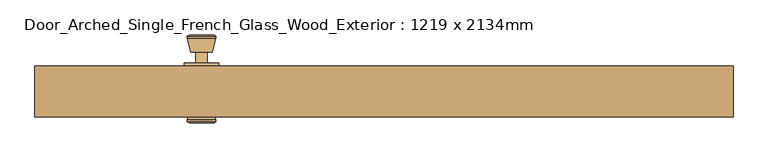
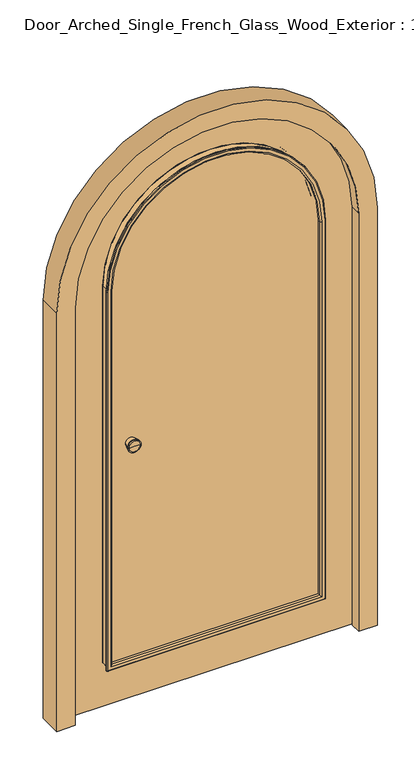
"""IFC4 building model written with IfcOpenShell, lengths in millimetres: door geometry, Door_Arched_Single_French_Glass_Wood_Exterior : 1219 x 2134mm."""

from ifc_helpers import new_model, si_unit, point, frame, frame_2d, origin, place, context, project, spatial, polyline, circle_curve, ellipse_curve, trimmed, segment, composite_curve, outline, extrude, source, transform, mapped, element, save
from ifc_brep_helpers import plane_surface, cylinder_surface, revolved_surface, advanced_brep


def door_arched_single_french_glass_wood_exterior_1219_x_2134mm_67be639c(model_context):
    return source(origin(), model_context, "Body", "SolidModel", [
        advanced_brep(
        [(-318.5, 5.7, 1050.0), (-328.5, 5.7, 1050.0), (-308.5, 5.7, 1050.0), (-298.0241324, 54.7, 1050.0), (-338.9758676, 54.7, 1050.0), (-318.5, 54.7, 1050.0), (-293.5, 52.8721319, 1050.0), (-343.5, 52.8721319, 1050.0), (-293.5, 49.4084537, 1050.0), (-343.5, 49.4084537, 1050.0), (-299.863764, 24.7, 1050.0), (-337.136236, 24.7, 1050.0), (-308.5, 24.7, 1050.0), (-328.5, 24.7, 1050.0)],
        [
            (0, 1),
            (1, 2, circle_curve(frame((-318.5, 5.7, 1050.0), z_axis=(0.0, -1.0, 0.0), x_axis=(-1.0, 0.0, 0.0)), 10.0)),
            (2, 0),
            (2, 1, circle_curve(frame((-318.5, 5.7, 1050.0), z_axis=(0.0, -1.0, 0.0), x_axis=(-1.0, 0.0, 0.0)), 10.0)),
            (3, 4, circle_curve(frame((-318.5, 54.7, 1050.0), z_axis=(0.0, 1.0, 0.0), x_axis=(-1.0, 0.0, 0.0)), 20.4758676)),
            (4, 5),
            (5, 3),
            (4, 3, circle_curve(frame((-318.5, 54.7, 1050.0), z_axis=(0.0, 1.0, 0.0), x_axis=(-1.0, 0.0, 0.0)), 20.4758676)),
            (6, 7, circle_curve(frame((-318.5, 52.8721319, 1050.0), z_axis=(0.0, 1.0, 0.0), x_axis=(-1.0, 0.0, 0.0)), 25.0)),
            (7, 4),
            (3, 6),
            (7, 6, circle_curve(frame((-318.5, 52.8721319, 1050.0), z_axis=(0.0, 1.0, 0.0), x_axis=(-1.0, 0.0, 0.0)), 25.0)),
            (8, 9, circle_curve(frame((-318.5, 49.4084537, 1050.0), z_axis=(0.0, 1.0, 0.0), x_axis=(-1.0, 0.0, 0.0)), 25.0)),
            (9, 7),
            (6, 8),
            (9, 8, circle_curve(frame((-318.5, 49.4084537, 1050.0), z_axis=(0.0, 1.0, 0.0), x_axis=(-1.0, 0.0, 0.0)), 25.0)),
            (10, 11, circle_curve(frame((-318.5, 24.7, 1050.0), z_axis=(0.0, 1.0, 0.0), x_axis=(-1.0, 0.0, 0.0)), 18.636236)),
            (11, 9),
            (8, 10),
            (11, 10, circle_curve(frame((-318.5, 24.7, 1050.0), z_axis=(0.0, 1.0, 0.0), x_axis=(-1.0, 0.0, 0.0)), 18.636236)),
            (12, 13, circle_curve(frame((-318.5, 24.7, 1050.0), z_axis=(0.0, 1.0, 0.0), x_axis=(-1.0, 0.0, 0.0)), 10.0)),
            (13, 11),
            (10, 12),
            (13, 12, circle_curve(frame((-318.5, 24.7, 1050.0), z_axis=(0.0, 1.0, 0.0), x_axis=(-1.0, 0.0, 0.0)), 10.0)),
            (1, 13),
            (12, 2),
        ],
        [
            plane_surface(frame((-318.5, 5.7, 1050.0), z_axis=(0.0, -1.0, 0.0), x_axis=(-1.0, 0.0, 0.0))),
            plane_surface(frame((-318.5, 54.7, 1050.0), z_axis=(0.0, 1.0, 0.0), x_axis=(-1.0, 0.0, 0.0))),
            revolved_surface(polyline([(-338.9758676, 54.7, 1050.0), (-343.5, 52.8721319, 1050.0)]), (-318.5, 5.7, 1050.0), (0.0, -1.0, 0.0)),
            cylinder_surface(frame((-318.5, 5.7, 1050.0), z_axis=(0.0, -1.0, 0.0), x_axis=(-1.0, 0.0, 0.0)), 25.0),
            revolved_surface(polyline([(-343.5, 49.4084537, 1050.0), (-337.136236, 24.7, 1050.0)]), (-318.5, 5.7, 1050.0), (0.0, -1.0, 0.0)),
            plane_surface(frame((-318.5, 24.7, 1050.0), z_axis=(0.0, -1.0, 0.0), x_axis=(-1.0, 0.0, 0.0))),
            cylinder_surface(frame((-318.5, 5.7, 1050.0), z_axis=(0.0, -1.0, 0.0), x_axis=(-1.0, 0.0, 0.0)), 10.0),
        ],
        [
            (0, [[1, 2, 3]]),
            (0, [[-3, 4, -1]]),
            (1, [[5, 6, 7]]),
            (1, [[8, -7, -6]]),
            (2, [[9, 10, -5, 11]]),
            (2, [[12, -11, -8, -10]]),
            (3, [[13, 14, -9, 15]]),
            (3, [[16, -15, -12, -14]]),
            (4, [[17, 18, -13, 19]]),
            (4, [[20, -19, -16, -18]]),
            (5, [[21, 22, -17, 23]]),
            (5, [[24, -23, -20, -22]]),
            (6, [[-2, 25, -21, 26]]),
            (6, [[-4, -26, -24, -25]]),
        ],
    ),
        extrude(outline(composite_curve([segment(trimmed(circle_curve(frame_2d((1050.0, -318.5)), 30.0), [point((1050.0, -348.5))], [point((1050.0, -288.5))], False, "CARTESIAN"), True, "CONTINUOUS"), segment(trimmed(circle_curve(frame_2d((1050.0, -318.5)), 30.0), [point((1050.0, -288.5))], [point((1050.0, -348.5))], False, "CARTESIAN"), True, "CONTINUOUS")], self_intersect=False)), frame((0.0, -0.3, 0.0), z_axis=(0.0, 1.0, 0.0), x_axis=(0.0, 0.0, 1.0)), (0.0, 0.0, 1.0), 6.0),
        advanced_brep(
        [(-318.5, -50.3, 1050.0), (-308.5, -50.3, 1050.0), (-328.5, -50.3, 1050.0), (-298.0241324, -99.3, 1050.0), (-318.5, -99.3, 1050.0), (-338.9758676, -99.3, 1050.0), (-293.5, -97.4721319, 1050.0), (-343.5, -97.4721319, 1050.0), (-293.5, -94.0084537, 1050.0), (-343.5, -94.0084537, 1050.0), (-299.863764, -69.3, 1050.0), (-337.136236, -69.3, 1050.0), (-308.5, -69.3, 1050.0), (-328.5, -69.3, 1050.0)],
        [
            (0, 1),
            (1, 2, circle_curve(frame((-318.5, -50.3, 1050.0), z_axis=(0.0, 1.0, 0.0), x_axis=(-1.0, 0.0, 0.0)), 10.0)),
            (2, 0),
            (2, 1, circle_curve(frame((-318.5, -50.3, 1050.0), z_axis=(0.0, 1.0, 0.0), x_axis=(-1.0, 0.0, 0.0)), 10.0)),
            (3, 4),
            (4, 5),
            (5, 3, circle_curve(frame((-318.5, -99.3, 1050.0), z_axis=(0.0, -1.0, 0.0), x_axis=(-1.0, 0.0, 0.0)), 20.4758676)),
            (3, 5, circle_curve(frame((-318.5, -99.3, 1050.0), z_axis=(0.0, -1.0, 0.0), x_axis=(-1.0, 0.0, 0.0)), 20.4758676)),
            (6, 3),
            (5, 7),
            (7, 6, circle_curve(frame((-318.5, -97.4721319, 1050.0), z_axis=(0.0, -1.0, 0.0), x_axis=(-1.0, 0.0, 0.0)), 25.0)),
            (6, 7, circle_curve(frame((-318.5, -97.4721319, 1050.0), z_axis=(0.0, -1.0, 0.0), x_axis=(-1.0, 0.0, 0.0)), 25.0)),
            (8, 6),
            (7, 9),
            (9, 8, circle_curve(frame((-318.5, -94.0084537, 1050.0), z_axis=(0.0, -1.0, 0.0), x_axis=(-1.0, 0.0, 0.0)), 25.0)),
            (8, 9, circle_curve(frame((-318.5, -94.0084537, 1050.0), z_axis=(0.0, -1.0, 0.0), x_axis=(-1.0, 0.0, 0.0)), 25.0)),
            (10, 8),
            (9, 11),
            (11, 10, circle_curve(frame((-318.5, -69.3, 1050.0), z_axis=(0.0, -1.0, 0.0), x_axis=(-1.0, 0.0, 0.0)), 18.636236)),
            (10, 11, circle_curve(frame((-318.5, -69.3, 1050.0), z_axis=(0.0, -1.0, 0.0), x_axis=(-1.0, 0.0, 0.0)), 18.636236)),
            (12, 10),
            (11, 13),
            (13, 12, circle_curve(frame((-318.5, -69.3, 1050.0), z_axis=(0.0, -1.0, 0.0), x_axis=(-1.0, 0.0, 0.0)), 10.0)),
            (12, 13, circle_curve(frame((-318.5, -69.3, 1050.0), z_axis=(0.0, -1.0, 0.0), x_axis=(-1.0, 0.0, 0.0)), 10.0)),
            (1, 12),
            (13, 2),
        ],
        [
            plane_surface(frame((-318.5, -50.3, 1050.0), z_axis=(0.0, 1.0, 0.0), x_axis=(-1.0, 0.0, 0.0))),
            plane_surface(frame((-318.5, -99.3, 1050.0), z_axis=(0.0, -1.0, 0.0), x_axis=(-1.0, 0.0, 0.0))),
            revolved_surface(polyline([(-338.9758676, -99.3, 1050.0), (-343.5, -97.4721319, 1050.0)]), (-318.5, -50.3, 1050.0), (0.0, 1.0, 0.0)),
            cylinder_surface(frame((-318.5, -50.3, 1050.0), z_axis=(0.0, 1.0, 0.0), x_axis=(-1.0, 0.0, 0.0)), 25.0),
            revolved_surface(polyline([(-343.5, -94.0084537, 1050.0), (-337.136236, -69.3, 1050.0)]), (-318.5, -50.3, 1050.0), (0.0, 1.0, 0.0)),
            plane_surface(frame((-318.5, -69.3, 1050.0), z_axis=(0.0, 1.0, 0.0), x_axis=(-1.0, 0.0, 0.0))),
            cylinder_surface(frame((-318.5, -50.3, 1050.0), z_axis=(0.0, 1.0, 0.0), x_axis=(-1.0, 0.0, 0.0)), 10.0),
        ],
        [
            (0, [[1, 2, 3]]),
            (0, [[-3, 4, -1]]),
            (1, [[5, 6, 7]]),
            (1, [[-6, -5, 8]]),
            (2, [[9, -7, 10, 11]]),
            (2, [[-10, -8, -9, 12]]),
            (3, [[13, -11, 14, 15]]),
            (3, [[-14, -12, -13, 16]]),
            (4, [[17, -15, 18, 19]]),
            (4, [[-18, -16, -17, 20]]),
            (5, [[21, -19, 22, 23]]),
            (5, [[-22, -20, -21, 24]]),
            (6, [[25, -23, 26, -2]]),
            (6, [[-26, -24, -25, -4]]),
        ],
    ),
        extrude(outline(composite_curve([segment(trimmed(circle_curve(frame_2d((1050.0, -318.5)), 30.0), [point((1050.0, -348.5))], [point((1050.0, -288.5))], False, "CARTESIAN"), True, "CONTINUOUS"), segment(trimmed(circle_curve(frame_2d((1050.0, -318.5)), 30.0), [point((1050.0, -288.5))], [point((1050.0, -348.5))], False, "CARTESIAN"), True, "CONTINUOUS")], self_intersect=False)), frame((0.0, -50.3, 0.0), z_axis=(0.0, 1.0, 0.0), x_axis=(0.0, 0.0, 1.0)), (0.0, 0.0, 1.0), 6.0),
        advanced_brep(
        [(539.1, -89.3, 0.0), (539.1, -47.3, 0.0), (561.1, -47.3, 0.0), (561.1, -0.3, 0.0), (609.6, -0.3, 0.0), (609.6, -89.3, 0.0), (609.6, -89.3, 1678.6), (-609.6, -89.3, 1678.6), (-609.6, -89.3, 0.0), (-539.1, -89.3, 0.0), (-539.1, -89.3, 1678.6), (539.1, -89.3, 1678.6), (609.6, -0.3, 1678.6), (561.1, -0.3, 1678.6), (-561.1, -0.3, 1678.6), (-561.1, -0.3, 0.0), (-609.6, -0.3, 0.0), (-609.6, -0.3, 1678.6), (561.1, -47.3, 1678.6), (539.1, -47.3, 1678.6), (-539.1, -47.3, 1678.6), (-539.1, -47.3, 0.0), (-561.1, -47.3, 0.0), (-561.1, -47.3, 1678.6)],
        [
            (0, 1),
            (1, 2),
            (2, 3),
            (3, 4),
            (4, 5),
            (5, 0),
            (5, 6),
            (6, 7, circle_curve(frame((0.0, -89.3, 1678.6), z_axis=(0.0, -1.0, 0.0), x_axis=(1.0, 0.0, 0.0)), 609.6)),
            (7, 8),
            (8, 9),
            (9, 10),
            (10, 11, circle_curve(frame((0.0, -89.3, 1678.6), z_axis=(0.0, 1.0, 0.0), x_axis=(1.0, 0.0, 0.0)), 539.1)),
            (11, 0),
            (4, 12),
            (12, 6),
            (3, 13),
            (13, 14, circle_curve(frame((0.0, -0.3, 1678.6), z_axis=(0.0, -1.0, 0.0), x_axis=(1.0, 0.0, 0.0)), 561.1)),
            (14, 15),
            (15, 16),
            (16, 17),
            (17, 12, circle_curve(frame((0.0, -0.3, 1678.6), z_axis=(0.0, 1.0, 0.0), x_axis=(1.0, 0.0, 0.0)), 609.6)),
            (2, 18),
            (18, 13),
            (1, 19),
            (19, 20, circle_curve(frame((0.0, -47.3, 1678.6), z_axis=(0.0, -1.0, 0.0), x_axis=(1.0, 0.0, 0.0)), 539.1)),
            (20, 21),
            (21, 22),
            (22, 23),
            (23, 18, circle_curve(frame((0.0, -47.3, 1678.6), z_axis=(0.0, 1.0, 0.0), x_axis=(1.0, 0.0, 0.0)), 561.1)),
            (11, 19),
            (9, 21),
            (20, 10),
            (8, 16),
            (15, 22),
            (7, 17),
            (14, 23),
        ],
        [
            plane_surface(frame((603.1, 9.1123976, 0.0), z_axis=(0.0, 0.0, -1.0), x_axis=(1.0, 0.0, 0.0))),
            plane_surface(frame((539.1, -89.3, 0.0), z_axis=(0.0, -1.0, 0.0), x_axis=(0.0, 0.0, 1.0))),
            plane_surface(frame((609.6, -89.3, 0.0), z_axis=(1.0, 0.0, 0.0), x_axis=(0.0, 0.0, 1.0))),
            plane_surface(frame((609.6, -0.3, 0.0), z_axis=(0.0, 1.0, 0.0), x_axis=(0.0, 0.0, 1.0))),
            plane_surface(frame((561.1, -0.3, 0.0), z_axis=(-1.0, 0.0, 0.0), x_axis=(0.0, 0.0, 1.0))),
            plane_surface(frame((561.1, -47.3, 0.0), z_axis=(0.0, 1.0, 0.0), x_axis=(0.0, 0.0, 1.0))),
            plane_surface(frame((539.1, -47.3, 0.0), z_axis=(-1.0, 0.0, 0.0), x_axis=(0.0, 0.0, 1.0))),
            plane_surface(frame((-539.1, -47.3, 1678.6), z_axis=(1.0, 0.0, 0.0), x_axis=(0.0, 0.0, -1.0))),
            plane_surface(frame((-603.1, 9.1123976, 0.0), z_axis=(0.0, 0.0, -1.0), x_axis=(-1.0, 0.0, 0.0))),
            plane_surface(frame((-609.6, -89.3, 1678.6), z_axis=(-1.0, 0.0, 0.0), x_axis=(0.0, 0.0, -1.0))),
            plane_surface(frame((-561.1, -0.3, 1678.6), z_axis=(1.0, 0.0, 0.0), x_axis=(0.0, 0.0, -1.0))),
            cylinder_surface(frame((0.0, -89.3, 1678.6), z_axis=(0.0, 1.0, 0.0), x_axis=(1.0, 0.0, 0.0)), 609.6),
            revolved_surface(polyline([(561.1, -0.29999999999999716, 1678.6), (561.1, -47.3, 1678.6)]), (0.0, -89.3, 1678.6), (0.0, 1.0, 0.0)),
            revolved_surface(polyline([(539.1, -47.3, 1678.6), (539.1, -89.3, 1678.6)]), (0.0, -89.3, 1678.6), (0.0, 1.0, 0.0)),
        ],
        [
            (0, [[1, 2, 3, 4, 5, 6]]),
            (1, [[7, 8, 9, 10, 11, 12, 13, -6]]),
            (2, [[14, 15, -7, -5]]),
            (3, [[16, 17, 18, 19, 20, 21, -14, -4]]),
            (4, [[22, 23, -16, -3]]),
            (5, [[24, 25, 26, 27, 28, 29, -22, -2]]),
            (6, [[-13, 30, -24, -1]]),
            (7, [[-11, 31, -26, 32]]),
            (8, [[-10, 33, -19, 34, -27, -31]]),
            (9, [[-20, -33, -9, 35]]),
            (10, [[-28, -34, -18, 36]]),
            (11, [[-35, -8, -15, -21]]),
            (12, [[-36, -17, -23, -29]]),
            (13, [[-32, -25, -30, -12]]),
        ],
    ),
        extrude(outline(composite_curve([segment(trimmed(circle_curve(frame_2d((1692.1, 0.0)), 253.5), [point((1896.740356, 149.6147543))], [point((1905.7961472, 136.3679092))], False, "CARTESIAN"), True, "CONTINUOUS"), segment(polyline([(1905.7961472, 136.3679092), (1768.2345335, 56.9466745)]), True, "CONTINUOUS"), segment(trimmed(circle_curve(frame_2d((1653.6, 0.0)), 128.0), [point((1768.2345335, 56.9466745))], [point((1768.2345335, -56.9466745))], False, "CARTESIAN"), True, "CONTINUOUS"), segment(polyline([(1768.2345335, -56.9466745), (1905.7961472, -136.3679092)]), True, "CONTINUOUS"), segment(trimmed(circle_curve(frame_2d((1692.1, 0.0)), 253.5), [point((1905.7961472, -136.3679092))], [point((1896.740356, -149.6147543))], False, "CARTESIAN"), True, "CONTINUOUS"), segment(polyline([(1896.740356, -149.6147543), (1760.2345335, -70.8030809)]), True, "CONTINUOUS"), segment(trimmed(circle_curve(frame_2d((1653.6, 0.0)), 128.0), [point((1760.2345335, -70.8030809))], [point((1661.6, -127.7497554))], False, "CARTESIAN"), True, "CONTINUOUS"), segment(polyline([(1661.6, -127.7497554), (1661.6, -408.1), (1645.6, -408.1), (1645.6, -128.0), (1273.5, -128.0), (1273.5, -408.1), (1257.5, -408.1), (1257.5, -128.0), (909.0, -128.0), (909.0, -408.1), (893.0, -408.1), (893.0, -128.0), (544.5, -128.0), (544.5, -408.1), (528.5, -408.1), (528.5, -128.0), (179.0, -128.0), (179.0, -112.0), (528.5, -112.0), (528.5, 112.0), (179.0, 112.0), (179.0, 128.0), (528.5, 128.0), (528.5, 408.1), (544.5, 408.1), (544.5, 128.0), (893.0, 128.0), (893.0, 408.1), (909.0, 408.1), (909.0, 128.0), (1257.5, 128.0), (1257.5, 408.1), (1273.5, 408.1), (1273.5, 128.0), (1645.6, 128.0), (1645.6, 408.1), (1661.6, 408.1), (1661.6, 127.7497554)]), True, "CONTINUOUS"), segment(trimmed(circle_curve(frame_2d((1653.6, 0.0)), 128.0), [point((1661.6, 127.7497554))], [point((1760.2345335, 70.8030809))], False, "CARTESIAN"), True, "CONTINUOUS"), segment(polyline([(1760.2345335, 70.8030809), (1896.740356, 149.6147543)]), True, "CONTINUOUS")], self_intersect=False), holes=[polyline([(893.0, -112.0), (893.0, 112.0), (544.5, 112.0), (544.5, -112.0), (893.0, -112.0)]), polyline([(1257.5, 112.0), (909.0, 112.0), (909.0, -112.0), (1257.5, -112.0), (1257.5, 112.0)]), composite_curve([segment(trimmed(circle_curve(frame_2d((1653.6, 0.0)), 112.0), [point((1661.6, -111.7139204))], [point((1661.6, 111.7139204))], True, "CARTESIAN"), True, "CONTINUOUS"), segment(polyline([(1661.6, 111.7139204), (1661.6, -111.7139204)]), True, "CONTINUOUS")], self_intersect=False), polyline([(1645.6, -112.0), (1645.6, 112.0), (1273.5, 112.0), (1273.5, -112.0), (1645.6, -112.0)])]), frame((0.0, -29.6874553, 0.0), z_axis=(0.0, 1.0, 0.0), x_axis=(0.0, 0.0, 1.0)), (0.0, 0.0, 1.0), 14.5359085),
        extrude(outline(composite_curve([segment(polyline([(4.0, 558.1), (1727.8950302, 558.1)]), True, "CONTINUOUS"), segment(trimmed(circle_curve(frame_2d((1678.6, 0.0)), 560.2727996), [point((1727.8950302, 558.1))], [point((1715.9714663, -559.0250294))], False, "CARTESIAN"), True, "CONTINUOUS"), segment(polyline([(1715.9714663, -559.0250294), (4.0, -559.0250294), (4.0, 558.1)]), True, "CONTINUOUS")], self_intersect=False), holes=[composite_curve([segment(polyline([(179.0, -408.1), (1692.1, -408.1)]), True, "CONTINUOUS"), segment(trimmed(circle_curve(frame_2d((1692.1, 0.0)), 408.1), [point((1692.1, -408.1))], [point((1692.1, 408.1))], True, "CARTESIAN"), True, "CONTINUOUS"), segment(polyline([(1692.1, 408.1), (179.0, 408.1), (179.0, -408.1)]), True, "CONTINUOUS")], self_intersect=False)]), frame((0.0, -44.3, 0.0), z_axis=(0.0, 1.0, 0.0), x_axis=(0.0, 0.0, 1.0)), (0.0, 0.0, 1.0), 44.0),
        extrude(outline(composite_curve([segment(polyline([(179.0, -408.1), (179.0, 408.1), (1692.1, 408.1)]), True, "CONTINUOUS"), segment(trimmed(circle_curve(frame_2d((1692.1, 0.0)), 408.1), [point((1692.1, 408.1))], [point((1692.1, -408.1))], False, "CARTESIAN"), True, "CONTINUOUS"), segment(polyline([(1692.1, -408.1), (179.0, -408.1)]), True, "CONTINUOUS")], self_intersect=False)), frame((0.0, -70.0, 0.0), z_axis=(0.0, 1.0, 0.0), x_axis=(0.0, 0.0, 1.0)), (0.0, 0.0, 1.0), 24.0),
        advanced_brep(
        [(-416.1, -84.0, 171.0), (-416.1, -84.0, 1692.1), (-416.1, -80.0, 1692.1), (-416.1, -80.0, 171.0), (-414.1, -86.0, 173.0), (-414.1, -86.0, 1692.1), (-396.1, -81.0, 191.0), (-396.1, -81.0, 1692.1), (-401.1, -86.0, 1692.1), (-401.1, -86.0, 186.0), (-396.1, -70.0, 191.0), (-396.1, -70.0, 1692.1), (-408.1, -80.0, 179.0), (-408.1, -80.0, 1692.1), (-408.1, -70.0, 1692.1), (-408.1, -70.0, 179.0), (416.1, -84.0, 1692.1), (416.1, -80.0, 1692.1), (414.1, -86.0, 1692.1), (414.1, -86.0, 173.0), (401.1, -86.0, 1692.1), (401.1, -86.0, 186.0), (396.1, -81.0, 1692.1), (396.1, -70.0, 1692.1), (408.1, -70.0, 1692.1), (408.1, -70.0, 179.0), (396.1, -70.0, 191.0), (408.1, -80.0, 1692.1), (416.1, -80.0, 171.0), (408.1, -80.0, 179.0), (416.1, -84.0, 171.0), (396.1, -81.0, 191.0)],
        [
            (0, 1),
            (1, 2),
            (2, 3),
            (3, 0),
            (4, 5),
            (5, 1, circle_curve(frame((-414.1, -84.0, 1692.1), z_axis=(0.0, 0.0, -1.0), x_axis=(-1.0, 0.0, 0.0)), 2.0)),
            (0, 4, ellipse_curve(frame((-414.1, -84.0, 173.0), z_axis=(-0.7071067811865475, 0.0, 0.7071067811865475), x_axis=(-0.7071067811865474, 0.0, -0.7071067811865476)), 2.8284271, 2.0)),
            (6, 7),
            (7, 8, circle_curve(frame((-401.1, -81.0, 1692.1), z_axis=(0.0, 0.0, -1.0), x_axis=(-1.0, 0.0, 0.0)), 5.0)),
            (8, 9),
            (9, 6, ellipse_curve(frame((-401.1, -81.0, 186.0), z_axis=(-0.7071067811865475, 0.0, 0.7071067811865475), x_axis=(-0.7071067811865474, 0.0, -0.7071067811865476)), 7.0710678, 5.0)),
            (10, 11),
            (11, 7),
            (6, 10),
            (12, 13),
            (13, 14),
            (14, 15),
            (15, 12),
            (16, 17),
            (17, 2, circle_curve(frame((0.0, -80.0, 1692.1), z_axis=(0.0, -1.0, 0.0), x_axis=(-1.0, 0.0, 0.0)), 416.1)),
            (1, 16, circle_curve(frame((0.0, -84.0, 1692.1), z_axis=(0.0, 1.0, 0.0), x_axis=(-1.0, 0.0, 0.0)), 416.1)),
            (18, 16, circle_curve(frame((414.1, -84.0, 1692.1), z_axis=(0.0, 0.0, 1.0), x_axis=(1.0, 0.0, 0.0)), 2.0)),
            (5, 18, circle_curve(frame((0.0, -86.0, 1692.1), z_axis=(0.0, 1.0, 0.0), x_axis=(-1.0, 0.0, 0.0)), 414.1)),
            (4, 19),
            (19, 18),
            (20, 21),
            (21, 9),
            (8, 20, circle_curve(frame((0.0, -86.0, 1692.1), z_axis=(0.0, 1.0, 0.0), x_axis=(-1.0, 0.0, 0.0)), 401.1)),
            (22, 20, circle_curve(frame((401.1, -81.0, 1692.1), z_axis=(0.0, 0.0, 1.0), x_axis=(1.0, 0.0, 0.0)), 5.0)),
            (7, 22, circle_curve(frame((0.0, -81.0, 1692.1), z_axis=(0.0, 1.0, 0.0), x_axis=(-1.0, 0.0, 0.0)), 396.1)),
            (23, 22),
            (11, 23, circle_curve(frame((0.0, -70.0, 1692.1), z_axis=(0.0, 1.0, 0.0), x_axis=(-1.0, 0.0, 0.0)), 396.1)),
            (24, 25),
            (25, 15),
            (14, 24, circle_curve(frame((0.0, -70.0, 1692.1), z_axis=(0.0, 1.0, 0.0), x_axis=(-1.0, 0.0, 0.0)), 408.1)),
            (10, 26),
            (26, 23),
            (27, 24),
            (13, 27, circle_curve(frame((0.0, -80.0, 1692.1), z_axis=(0.0, 1.0, 0.0), x_axis=(-1.0, 0.0, 0.0)), 408.1)),
            (17, 28),
            (28, 3),
            (12, 29),
            (29, 27),
            (16, 30),
            (30, 28),
            (19, 30, ellipse_curve(frame((414.1, -84.0, 173.0), z_axis=(0.7071067811865475, 0.0, 0.7071067811865475), x_axis=(-0.7071067811865474, 0.0, 0.7071067811865476)), 2.8284271, 2.0)),
            (22, 31),
            (31, 21, ellipse_curve(frame((401.1, -81.0, 186.0), z_axis=(0.7071067811865475, 0.0, 0.7071067811865475), x_axis=(-0.7071067811865474, 0.0, 0.7071067811865476)), 7.0710678, 5.0)),
            (26, 31),
            (29, 25),
            (30, 0),
            (31, 6),
        ],
        [
            plane_surface(frame((-416.1, -80.0, 171.0), z_axis=(-1.0, 0.0, 0.0), x_axis=(0.0, 0.0, 1.0))),
            cylinder_surface(frame((-414.1, -84.0, 179.0), z_axis=(0.0, 0.0, -1.0), x_axis=(-1.0, 0.0, 0.0)), 2.0),
            cylinder_surface(frame((-401.1, -81.0, 179.0), z_axis=(0.0, 0.0, -1.0), x_axis=(-1.0, 0.0, 0.0)), 5.0),
            plane_surface(frame((-396.1, -81.0, 191.0), z_axis=(1.0, 0.0, 0.0), x_axis=(0.0, 0.0, 1.0))),
            plane_surface(frame((-408.1, -70.0, 179.0), z_axis=(-1.0, 0.0, 0.0), x_axis=(0.0, 0.0, 1.0))),
            cylinder_surface(frame((0.0, -80.0, 1692.1), z_axis=(0.0, -1.0, 0.0), x_axis=(-1.0, 0.0, 0.0)), 416.1),
            revolved_surface(trimmed(ellipse_curve(frame((-414.1, -84.0, 1692.1), z_axis=(0.0, 0.0, 1.0), x_axis=(-1.0, 0.0, 0.0)), 2.0, 2.0), [point((-416.1, -84.0, 1692.1))], [point((-414.1, -86.0, 1692.1))], True, "CARTESIAN"), (0.0, -80.0, 1692.1), (0.0, -1.0, 0.0)),
            plane_surface(frame((0.0, -86.0, 1692.1), z_axis=(0.0, -1.0, 0.0), x_axis=(-1.0, 0.0, 0.0))),
            revolved_surface(trimmed(ellipse_curve(frame((-401.1, -81.0, 1692.1), z_axis=(0.0, 0.0, 1.0), x_axis=(-1.0, 0.0, 0.0)), 5.0, 5.0), [point((-401.1, -86.0, 1692.1))], [point((-396.1, -81.0, 1692.1))], True, "CARTESIAN"), (0.0, -80.0, 1692.1), (0.0, -1.0, 0.0)),
            revolved_surface(polyline([(-396.1, -81.0, 1692.1), (-396.1, -70.0, 1692.1)]), (0.0, -80.0, 1692.1), (0.0, -1.0, 0.0)),
            plane_surface(frame((0.0, -70.0, 1692.1), z_axis=(0.0, 1.0, 0.0), x_axis=(-1.0, 0.0, 0.0))),
            cylinder_surface(frame((0.0, -80.0, 1692.1), z_axis=(0.0, -1.0, 0.0), x_axis=(-1.0, 0.0, 0.0)), 408.1),
            plane_surface(frame((0.0, -80.0, 1692.1), z_axis=(0.0, 1.0, 0.0), x_axis=(-1.0, 0.0, 0.0))),
            plane_surface(frame((416.1, -80.0, 1692.1), z_axis=(1.0, 0.0, 0.0), x_axis=(0.0, 0.0, -1.0))),
            cylinder_surface(frame((414.1, -84.0, 1692.1), z_axis=(0.0, 0.0, 1.0), x_axis=(1.0, 0.0, 0.0)), 2.0),
            cylinder_surface(frame((401.1, -81.0, 1692.1), z_axis=(0.0, 0.0, 1.0), x_axis=(1.0, 0.0, 0.0)), 5.0),
            plane_surface(frame((396.1, -81.0, 1692.1), z_axis=(-1.0, 0.0, 0.0), x_axis=(0.0, 0.0, -1.0))),
            plane_surface(frame((408.1, -70.0, 1692.1), z_axis=(1.0, 0.0, 0.0), x_axis=(0.0, 0.0, -1.0))),
            plane_surface(frame((416.1, -80.0, 171.0), z_axis=(0.0, 0.0, -1.0), x_axis=(-1.0, 0.0, 0.0))),
            cylinder_surface(frame((408.1, -84.0, 173.0), z_axis=(1.0, 0.0, 0.0), x_axis=(0.0, 0.0, -1.0)), 2.0),
            cylinder_surface(frame((408.1, -81.0, 186.0), z_axis=(1.0, 0.0, 0.0), x_axis=(0.0, 0.0, -1.0)), 5.0),
            plane_surface(frame((396.1, -81.0, 191.0), z_axis=(0.0, 0.0, 1.0), x_axis=(-1.0, 0.0, 0.0))),
            plane_surface(frame((408.1, -70.0, 179.0), z_axis=(0.0, 0.0, -1.0), x_axis=(-1.0, 0.0, 0.0))),
        ],
        [
            (0, [[1, 2, 3, 4]]),
            (1, [[5, 6, -1, 7]]),
            (2, [[8, 9, 10, 11]]),
            (3, [[12, 13, -8, 14]]),
            (4, [[15, 16, 17, 18]]),
            (5, [[19, 20, -2, 21]]),
            (6, [[22, -21, -6, 23]]),
            (7, [[-23, -5, 24, 25], [26, 27, -10, 28]]),
            (8, [[29, -28, -9, 30]]),
            (9, [[31, -30, -13, 32]]),
            (10, [[33, 34, -17, 35], [-32, -12, 36, 37]]),
            (11, [[38, -35, -16, 39]]),
            (12, [[40, 41, -3, -20], [-39, -15, 42, 43]]),
            (13, [[44, 45, -40, -19]]),
            (14, [[-25, 46, -44, -22]]),
            (15, [[47, 48, -26, -29]]),
            (16, [[-37, 49, -47, -31]]),
            (17, [[-43, 50, -33, -38]]),
            (18, [[51, -4, -41, -45]]),
            (19, [[-24, -7, -51, -46]]),
            (20, [[52, -11, -27, -48]]),
            (21, [[-36, -14, -52, -49]]),
            (22, [[-42, -18, -34, -50]]),
        ],
    ),
        advanced_brep(
        [(416.1, -32.0, 171.0), (416.1, -32.0, 1692.1), (416.1, -36.0, 1692.1), (416.1, -36.0, 171.0), (414.1, -30.0, 173.0), (414.1, -30.0, 1692.1), (396.1, -35.0, 191.0), (396.1, -35.0, 1692.1), (401.1, -30.0, 1692.1), (401.1, -30.0, 186.0), (396.1, -46.0, 191.0), (396.1, -46.0, 1692.1), (408.1, -36.0, 179.0), (408.1, -36.0, 1692.1), (408.1, -46.0, 1692.1), (408.1, -46.0, 179.0), (-416.1, -32.0, 1692.1), (-416.1, -36.0, 1692.1), (-414.1, -30.0, 1692.1), (-414.1, -30.0, 173.0), (-401.1, -30.0, 1692.1), (-401.1, -30.0, 186.0), (-396.1, -35.0, 1692.1), (-396.1, -46.0, 1692.1), (-408.1, -46.0, 1692.1), (-408.1, -46.0, 179.0), (-396.1, -46.0, 191.0), (-408.1, -36.0, 1692.1), (-416.1, -36.0, 171.0), (-408.1, -36.0, 179.0), (-416.1, -32.0, 171.0), (-396.1, -35.0, 191.0)],
        [
            (0, 1),
            (1, 2),
            (2, 3),
            (3, 0),
            (4, 5),
            (5, 1, circle_curve(frame((414.1, -32.0, 1692.1), z_axis=(0.0, 0.0, -1.0), x_axis=(1.0, 0.0, 0.0)), 2.0)),
            (0, 4, ellipse_curve(frame((414.1, -32.0, 173.0), z_axis=(0.7071067811865475, 0.0, 0.7071067811865475), x_axis=(0.7071067811865474, 0.0, -0.7071067811865476)), 2.8284271, 2.0)),
            (6, 7),
            (7, 8, circle_curve(frame((401.1, -35.0, 1692.1), z_axis=(0.0, 0.0, -1.0), x_axis=(1.0, 0.0, 0.0)), 5.0)),
            (8, 9),
            (9, 6, ellipse_curve(frame((401.1, -35.0, 186.0), z_axis=(0.7071067811865475, 0.0, 0.7071067811865475), x_axis=(0.7071067811865474, 0.0, -0.7071067811865476)), 7.0710678, 5.0)),
            (10, 11),
            (11, 7),
            (6, 10),
            (12, 13),
            (13, 14),
            (14, 15),
            (15, 12),
            (16, 17),
            (17, 2, circle_curve(frame((0.0, -36.0, 1692.1), z_axis=(0.0, 1.0, 0.0), x_axis=(1.0, 0.0, 0.0)), 416.1)),
            (1, 16, circle_curve(frame((0.0, -32.0, 1692.1), z_axis=(0.0, -1.0, 0.0), x_axis=(1.0, 0.0, 0.0)), 416.1)),
            (18, 16, circle_curve(frame((-414.1, -32.0, 1692.1), z_axis=(0.0, 0.0, 1.0), x_axis=(-1.0, 0.0, 0.0)), 2.0)),
            (5, 18, circle_curve(frame((0.0, -30.0, 1692.1), z_axis=(0.0, -1.0, 0.0), x_axis=(1.0, 0.0, 0.0)), 414.1)),
            (4, 19),
            (19, 18),
            (20, 21),
            (21, 9),
            (8, 20, circle_curve(frame((0.0, -30.0, 1692.1), z_axis=(0.0, -1.0, 0.0), x_axis=(1.0, 0.0, 0.0)), 401.1)),
            (22, 20, circle_curve(frame((-401.1, -35.0, 1692.1), z_axis=(0.0, 0.0, 1.0), x_axis=(-1.0, 0.0, 0.0)), 5.0)),
            (7, 22, circle_curve(frame((0.0, -35.0, 1692.1), z_axis=(0.0, -1.0, 0.0), x_axis=(1.0, 0.0, 0.0)), 396.1)),
            (23, 22),
            (11, 23, circle_curve(frame((0.0, -46.0, 1692.1), z_axis=(0.0, -1.0, 0.0), x_axis=(1.0, 0.0, 0.0)), 396.1)),
            (24, 25),
            (25, 15),
            (14, 24, circle_curve(frame((0.0, -46.0, 1692.1), z_axis=(0.0, -1.0, 0.0), x_axis=(1.0, 0.0, 0.0)), 408.1)),
            (10, 26),
            (26, 23),
            (27, 24),
            (13, 27, circle_curve(frame((0.0, -36.0, 1692.1), z_axis=(0.0, -1.0, 0.0), x_axis=(1.0, 0.0, 0.0)), 408.1)),
            (17, 28),
            (28, 3),
            (12, 29),
            (29, 27),
            (16, 30),
            (30, 28),
            (19, 30, ellipse_curve(frame((-414.1, -32.0, 173.0), z_axis=(-0.7071067811865475, 0.0, 0.7071067811865475), x_axis=(0.7071067811865474, 0.0, 0.7071067811865476)), 2.8284271, 2.0)),
            (22, 31),
            (31, 21, ellipse_curve(frame((-401.1, -35.0, 186.0), z_axis=(-0.7071067811865475, 0.0, 0.7071067811865475), x_axis=(0.7071067811865474, 0.0, 0.7071067811865476)), 7.0710678, 5.0)),
            (26, 31),
            (29, 25),
            (30, 0),
            (31, 6),
        ],
        [
            plane_surface(frame((416.1, -36.0, 171.0), z_axis=(1.0, 0.0, 0.0), x_axis=(0.0, 0.0, 1.0))),
            cylinder_surface(frame((414.1, -32.0, 179.0), z_axis=(0.0, 0.0, -1.0), x_axis=(1.0, 0.0, 0.0)), 2.0),
            cylinder_surface(frame((401.1, -35.0, 179.0), z_axis=(0.0, 0.0, -1.0), x_axis=(1.0, 0.0, 0.0)), 5.0),
            plane_surface(frame((396.1, -35.0, 191.0), z_axis=(-1.0, 0.0, 0.0), x_axis=(0.0, 0.0, 1.0))),
            plane_surface(frame((408.1, -46.0, 179.0), z_axis=(1.0, 0.0, 0.0), x_axis=(0.0, 0.0, 1.0))),
            cylinder_surface(frame((0.0, -36.0, 1692.1), z_axis=(0.0, 1.0, 0.0), x_axis=(1.0, 0.0, 0.0)), 416.1),
            revolved_surface(trimmed(ellipse_curve(frame((414.1, -32.0, 1692.1), z_axis=(0.0, 0.0, 1.0), x_axis=(1.0, 0.0, 0.0)), 2.0, 2.0), [point((416.1, -32.0, 1692.1))], [point((414.1, -30.0, 1692.1))], True, "CARTESIAN"), (0.0, -36.0, 1692.1), (0.0, 1.0, 0.0)),
            plane_surface(frame((0.0, -30.0, 1692.1), z_axis=(0.0, 1.0, 0.0), x_axis=(1.0, 0.0, 0.0))),
            revolved_surface(trimmed(ellipse_curve(frame((401.1, -35.0, 1692.1), z_axis=(0.0, 0.0, 1.0), x_axis=(1.0, 0.0, 0.0)), 5.0, 5.0), [point((401.1, -30.0, 1692.1))], [point((396.1, -35.0, 1692.1))], True, "CARTESIAN"), (0.0, -36.0, 1692.1), (0.0, 1.0, 0.0)),
            revolved_surface(polyline([(396.1, -35.0, 1692.1), (396.1, -46.0, 1692.1)]), (0.0, -36.0, 1692.1), (0.0, 1.0, 0.0)),
            plane_surface(frame((0.0, -46.0, 1692.1), z_axis=(0.0, -1.0, 0.0), x_axis=(1.0, 0.0, 0.0))),
            cylinder_surface(frame((0.0, -36.0, 1692.1), z_axis=(0.0, 1.0, 0.0), x_axis=(1.0, 0.0, 0.0)), 408.1),
            plane_surface(frame((0.0, -36.0, 1692.1), z_axis=(0.0, -1.0, 0.0), x_axis=(1.0, 0.0, 0.0))),
            plane_surface(frame((-416.1, -36.0, 1692.1), z_axis=(-1.0, 0.0, 0.0), x_axis=(0.0, 0.0, -1.0))),
            cylinder_surface(frame((-414.1, -32.0, 1692.1), z_axis=(0.0, 0.0, 1.0), x_axis=(-1.0, 0.0, 0.0)), 2.0),
            cylinder_surface(frame((-401.1, -35.0, 1692.1), z_axis=(0.0, 0.0, 1.0), x_axis=(-1.0, 0.0, 0.0)), 5.0),
            plane_surface(frame((-396.1, -35.0, 1692.1), z_axis=(1.0, 0.0, 0.0), x_axis=(0.0, 0.0, -1.0))),
            plane_surface(frame((-408.1, -46.0, 1692.1), z_axis=(-1.0, 0.0, 0.0), x_axis=(0.0, 0.0, -1.0))),
            plane_surface(frame((-416.1, -36.0, 171.0), z_axis=(0.0, 0.0, -1.0), x_axis=(1.0, 0.0, 0.0))),
            cylinder_surface(frame((-408.1, -32.0, 173.0), z_axis=(-1.0, 0.0, 0.0), x_axis=(0.0, 0.0, -1.0)), 2.0),
            cylinder_surface(frame((-408.1, -35.0, 186.0), z_axis=(-1.0, 0.0, 0.0), x_axis=(0.0, 0.0, -1.0)), 5.0),
            plane_surface(frame((-396.1, -35.0, 191.0), z_axis=(0.0, 0.0, 1.0), x_axis=(1.0, 0.0, 0.0))),
            plane_surface(frame((-408.1, -46.0, 179.0), z_axis=(0.0, 0.0, -1.0), x_axis=(1.0, 0.0, 0.0))),
        ],
        [
            (0, [[1, 2, 3, 4]]),
            (1, [[5, 6, -1, 7]]),
            (2, [[8, 9, 10, 11]]),
            (3, [[12, 13, -8, 14]]),
            (4, [[15, 16, 17, 18]]),
            (5, [[19, 20, -2, 21]]),
            (6, [[22, -21, -6, 23]]),
            (7, [[-23, -5, 24, 25], [26, 27, -10, 28]]),
            (8, [[29, -28, -9, 30]]),
            (9, [[31, -30, -13, 32]]),
            (10, [[33, 34, -17, 35], [-32, -12, 36, 37]]),
            (11, [[38, -35, -16, 39]]),
            (12, [[40, 41, -3, -20], [-39, -15, 42, 43]]),
            (13, [[44, 45, -40, -19]]),
            (14, [[-25, 46, -44, -22]]),
            (15, [[47, 48, -26, -29]]),
            (16, [[-37, 49, -47, -31]]),
            (17, [[-43, 50, -33, -38]]),
            (18, [[51, -4, -41, -45]]),
            (19, [[-24, -7, -51, -46]]),
            (20, [[52, -11, -27, -48]]),
            (21, [[-36, -14, -52, -49]]),
            (22, [[-42, -18, -34, -50]]),
        ],
    ),
    ])


if __name__ == "__main__":
    model = new_model("IFC4")
    model_context = context("Model", 3, world=origin())
    ifc_project = project(units=[si_unit("LENGTHUNIT", "METRE", prefix="MILLI")], contexts=[model_context])
    site = spatial("IfcSite", under=ifc_project)
    building = spatial("IfcBuilding", under=site)
    placement = place(None, origin())
    door_arched_single_french_glass_wood_exterior_1219_x_2134mm_shape = door_arched_single_french_glass_wood_exterior_1219_x_2134mm_67be639c(model_context)
    element("IfcDoor", 1, ObjectType="Door_Arched_Single_French_Glass_Wood_Exterior : 1219 x 2134mm", at=placement, inside=building, context=model_context, shape_type="MappedRepresentation", body=[
        mapped(door_arched_single_french_glass_wood_exterior_1219_x_2134mm_shape, transform((0.0, 0.0, 0.0), x_axis=(1.0, 0.0, 0.0), y_axis=(0.0, 1.0, 0.0), z_axis=(0.0, 0.0, 1.0))),
    ])
    save(model, "model.ifc")

# Revit data of these elements
# Type "Door_Arched_Single_French_Glass_Wood_Exterior : 1219 x 2134mm"
#   Type Mark = "12"
#   Type Comments = "External Single"
#   Operation = "SingleSwingRight"
#   Keynote = "L20"
#   Analytic Construction = "<None>"
#   Wrap Layers (Int) from Ext = 0' - 6.98819"
#   Wrap Layers (Ext) from Ext = 0' - 4.03543"
#   Thickness = 0' - 1.73228"
#   Stile Shutting = 0' - 5.90551"
#   Stile - Top Rail = 0' - 5.90551"
#   Stile - Hanging = 0' - 5.90551"
#   Stile - Bottom Rail = 0' - 6.88976"
#   Rough Width = 4' - 0"
#   Rough Height = 7' - 0"
#   O/A Frame Width = 0' - 2.51969"
#   Handle Z Distance = 3' - 5.33858"
#   Glazing Thickness = 0' - 0.94488"
#   Glazing Bar Thickness = 0' - 0.7874"
#   FrameWidth = 0' - 1.65354"
#   FrameOffset - External = 0' - 0.98425"
#   FrameDepth = 0' - 3.50394"
#   Door Panel Width = 3' - 7.94488"
#   Handle X Distance = 0' - 2.95276"
#   Height = 7' - 0"
#   Structural Tolerance = 0' - 0.25591"
#   Tolerance = 0' - 0.11811"
#   Undercut = 0' - 0.15748"
#   Width = 4' - 0"
#   Door Panel Thickness = 0' - 1.73228"
#   Door Panel Height = 6' - 9.81496"
#   Cavity Closer Width = 0' - 1.9685"
#   Cavity Closer Offset from Ext = 0' - 4.03543"
#   Cavity Closer Depth = 0' - 3.34646"
#   Vis - Ironmongery = yes
#   Vis - Cavity Closers = yes
#   Define Thermal Properties by = 1
#   Material Glass = Door - Glazing
#   Handle Style = element 451349
#   Material Door = Door - Panel
#   Material Frame = BROWN
#   Material Ironmongery = Door - Handle
#   Function = (empty or 0)
#   Wall Closure = (empty or 0)
#   Assembly Code = ""
# Element 1 (IfcDoor, "Door_Arched_Single_French_Glass_Wood_Exterior : 1219 x 2134mm")
#   Materials on its faces: "Door - Panel", "Door - Handle", "BROWN", "Door - Glazing"
# Materials
#   "Door - Glazing": colour RGB 218 227 224, transparency 0.85
#   "Door - Panel": class "Wood", colour RGB 210 159 95, transparency 0, Cost = 0
#   "BROWN": class "Generic", colour RGB 120 120 120, transparency 0, Cost = 0
#   "Door - Handle": colour RGB 0 0 0, transparency 0, Keynote = "P21"
